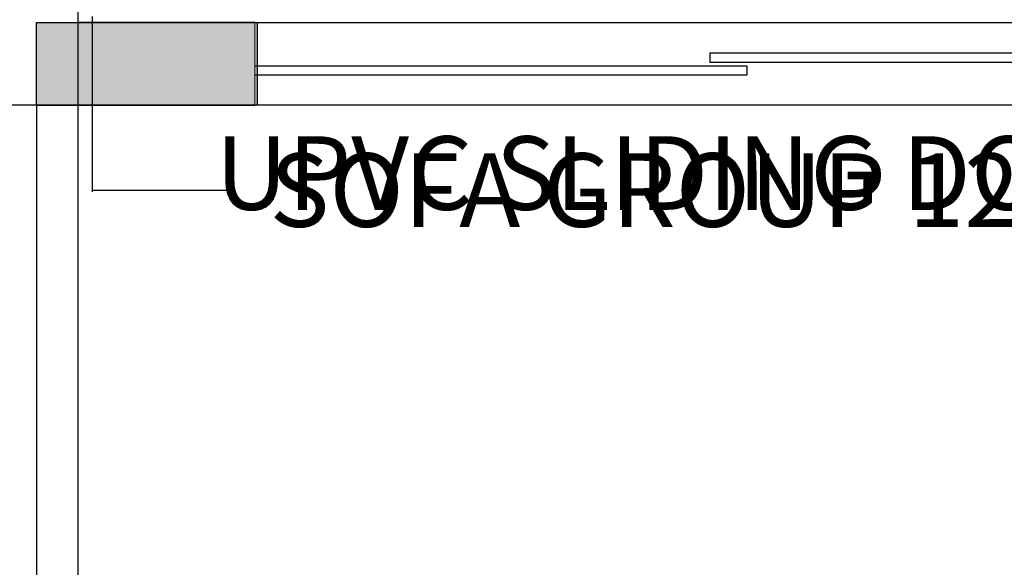
# Model space of a CAD drawing. Units: inches. Extents: x -48 to 50072, y 0 to 21068.
# Tile 47 of 75: x 16 to 123, y 628 to 687. Entities that reach past the tile are written whole.
import ezdxf

# ---------------------------------------------------------------- set-up
doc = ezdxf.new("R2010")
doc.units = ezdxf.units.IN
doc.header["$MEASUREMENT"] = 0
doc.linetypes.add('ACAD_ISO02W100', pattern=[15, 12, -3])
for name, color, linetype, lineweight in [('A-ANNO-DIMS', 2, 'Continuous', 18), ('A-ANNO-TEXT', 7, 'Continuous', 18), ('A-COLS', 1, 'Continuous', 35), ('A-DOOR', 4, 'Continuous', 18), ('A-WALL', 7, 'Continuous', 35), ('C-PROP', 7, 'Continuous', 25), ('C-PROP-REF', 32, 'ACAD_ISO02W100', 13)]:
    doc.layers.add(name, color=color, linetype=linetype, lineweight=lineweight)
doc.layers.add('Layer3', color=176, linetype='Continuous')
doc.styles.get("Standard").update_dxf_attribs({"font": 'arial.ttf'})
doc.dimstyles.get("Standard").update_dxf_attribs({"dimtxt": 8, "dimasz": 0.18, "dimexe": 0.18, "dimexo": 0.0625, "dimgap": 0.09, "dimtad": 0, "dimtih": 1, "dimtoh": 1, "dimdec": 1, "dimzin": 0, "dimdsep": 46, "dimlunit": 4, "dimtxsty": 'Standard', "dimblk": 'ARCHTICK', "dimcen": 0.09, "dimadec": 0, "dimazin": 0, "dimtfac": 1, "dimtdec": 1, "dimtofl": 0, "dimtmove": 0, "dimatfit": 3, "dimldrblk": 'ARCHTICK', "dimfxl": 1, "dimtolj": 1, "dimtzin": 0, "dimarcsym": 0})

# ---------------------------------------------------------------- blocks, each defined once
blk = doc.blocks.new('bnniku')
at = {"layer": 'Defpoints'}
h = blk.add_hatch(color=256, dxfattribs=at)
h.dxf.hatch_style = 1
h.paths.add_polyline_path([(767.55, 1114.04), (758.55, 1114.04), (758.55, 1090.04), (767.55, 1090.04)])
for p, q in [((758.55, 1114.04), (767.55, 1114.04)), ((758.55, 1090.04), (758.55, 1114.04)), ((767.55, 1114.04), (767.55, 1090.04)), ((767.55, 1090.04), (758.55, 1090.04))]:
    blk.add_line(p, q, dxfattribs=at)
blk = doc.blocks.new('fdsghhhhhhygr')
for p, q in [((41.77, 686.77), (41.77, 677.77)), ((144.77, 677.77), (144.77, 686.77))]:
    blk.add_line(p, q)
at = {"layer": 'Defpoints'}
for p, q in [((91.27, 683.47), (144.77, 683.47)), ((91.27, 683.47), (91.27, 682.47)), ((41.77, 682.07), (95.27, 682.07)), ((91.27, 682.47), (144.77, 682.47)), ((95.27, 682.07), (95.27, 681.07)), ((41.77, 681.07), (95.27, 681.07))]:
    blk.add_line(p, q, dxfattribs=at)
at = {"layer": 'Layer3'}
for p, q in [((41.77, 686.77), (144.77, 686.77)), ((144.77, 677.77), (41.77, 677.77))]:
    blk.add_line(p, q, dxfattribs=at)
blk = doc.blocks.new('_ArchTick')
at = {"color": 0, "linetype": 'ByBlock', "const_width": 0.15}
blk.add_lwpolyline([(-0.5, -0.5), (0.5, 0.5)], dxfattribs=at)
blk = doc.blocks.new('*D104')
at = {"layer": 'A-ANNO-DIMS', "color": 0, "lineweight": -2, "transparency": 16777216}
for p, q in [((51.57, 714.9), (55.29, 714.9)), ((55.11, 714.9), (55.11, 707.12)), ((55.11, 690.9), (55.11, 698.67)), ((51.57, 690.9), (55.29, 690.9))]:
    blk.add_line(p, q, dxfattribs=at)
at = {"layer": 'Defpoints', "color": 0, "transparency": 16777216}
for p in [(51.51, 714.9), (55.11, 714.9), (51.51, 690.9)]:
    blk.add_point(p, dxfattribs=at)
at = {"layer": 'A-ANNO-DIMS', "color": 0, "lineweight": -2, "transparency": 16777216, "xscale": 0.18, "yscale": 0.18, "zscale": 0.18}
for p, rotation in [((55.11, 714.9), 90), ((55.11, 690.9), 270)]:
    blk.add_blockref('_ArchTick', p, dxfattribs=dict(at, rotation=rotation))
at = {"layer": 'A-ANNO-DIMS', "color": 0, "transparency": 16777216, "insert": (55.11, 702.9), "char_height": 8, "attachment_point": 5}
blk.add_mtext('\\A1;SIDE TABLE 24', dxfattribs=at)
blk = doc.blocks.new('*D108')
at = {"layer": 'A-ANNO-DIMS', "color": 0, "lineweight": -2, "transparency": 16777216}
for p, q in [((24.1, 687.42), (24.1, 668.37)), ((150.3, 687.42), (150.3, 668.37)), ((24.1, 668.55), (39.48, 668.55)), ((150.3, 668.55), (134.91, 668.55))]:
    blk.add_line(p, q, dxfattribs=at)
at = {"layer": 'Defpoints', "color": 0, "transparency": 16777216}
for p in [(24.1, 687.48), (150.3, 687.48), (24.1, 668.55)]:
    blk.add_point(p, dxfattribs=at)
at = {"layer": 'A-ANNO-DIMS', "color": 0, "lineweight": -2, "transparency": 16777216, "xscale": 0.18, "yscale": 0.18, "zscale": 0.18, "rotation": 180}
blk.add_blockref('_ArchTick', (24.1, 668.55), dxfattribs=at)
at = {"layer": 'A-ANNO-DIMS', "color": 0, "lineweight": -2, "transparency": 16777216, "xscale": 0.18, "yscale": 0.18, "zscale": 0.18}
blk.add_blockref('_ArchTick', (150.3, 668.55), dxfattribs=at)
at = {"layer": 'A-ANNO-DIMS', "color": 0, "transparency": 16777216, "insert": (87.2, 668.55), "char_height": 8, "attachment_point": 5}
blk.add_mtext('\\A1;SOFA GROUP 126', dxfattribs=at)
blk = doc.blocks.new('*D116')
at = {"layer": 'A-ANNO-DIMS', "color": 0, "lineweight": -2, "transparency": 16777216}
for p, q in [((18.02, 677.71), (18.02, 165.94)), ((216.02, 677.71), (216.02, 165.94)), ((18.02, 166.12), (108.46, 166.12)), ((216.02, 166.12), (125.58, 166.12))]:
    blk.add_line(p, q, dxfattribs=at)
at = {"layer": 'Defpoints', "color": 0, "transparency": 16777216}
for p in [(18.02, 677.77), (216.02, 677.77), (216.02, 166.12)]:
    blk.add_point(p, dxfattribs=at)
at = {"layer": 'A-ANNO-DIMS', "color": 0, "lineweight": -2, "transparency": 16777216, "xscale": 0.18, "yscale": 0.18, "zscale": 0.18, "rotation": 180}
blk.add_blockref('_ArchTick', (18.02, 166.12), dxfattribs=at)
at = {"layer": 'A-ANNO-DIMS', "color": 0, "lineweight": -2, "transparency": 16777216, "xscale": 0.18, "yscale": 0.18, "zscale": 0.18}
blk.add_blockref('_ArchTick', (216.02, 166.12), dxfattribs=at)
at = {"layer": 'A-ANNO-DIMS', "color": 0, "transparency": 16777216, "insert": (117.02, 166.12), "char_height": 8, "attachment_point": 5}
blk.add_mtext('\\A1;198', dxfattribs=at)
blk = doc.blocks.new('*D127')
at = {"layer": 'A-ANNO-DIMS', "color": 0, "lineweight": -2, "transparency": 16777216}
for p, q in [((215.95, 677.77), (-34.61, 677.77)), ((-34.43, 677.77), (-34.43, 587.45)), ((-34.43, 488.77), (-34.43, 579.1)), ((215.95, 488.77), (-34.61, 488.77))]:
    blk.add_line(p, q, dxfattribs=at)
at = {"layer": 'Defpoints', "color": 0, "transparency": 16777216}
for p in [(-34.43, 677.77), (216.02, 677.77), (216.02, 488.77)]:
    blk.add_point(p, dxfattribs=at)
at = {"layer": 'A-ANNO-DIMS', "color": 0, "lineweight": -2, "transparency": 16777216, "xscale": 0.18, "yscale": 0.18, "zscale": 0.18}
for p, rotation in [((-34.43, 677.77), 90), ((-34.43, 488.77), 270)]:
    blk.add_blockref('_ArchTick', p, dxfattribs=dict(at, rotation=rotation))
at = {"layer": 'A-ANNO-DIMS', "color": 0, "transparency": 16777216, "insert": (-34.43, 583.27), "char_height": 8, "attachment_point": 5}
blk.add_mtext('\\A1;189', dxfattribs=at)

msp = doc.modelspace()

# ---------------------------------------------------------------- linework, layer by layer
at = {"layer": 'A-WALL'}
for p, q in [((41.766, 686.775), (22.517, 686.775)), ((41.766, 677.775), (18.017, 677.775))]:
    msp.add_line(p, q, dxfattribs=at)
at = {"layer": 'C-PROP'}
msp.add_line((22.517, 860.775), (22.517, 223.075), dxfattribs=at)
at = {"layer": 'C-PROP-REF'}
msp.add_line((18.017, 1166.275), (18.017, 214.075), dxfattribs=at)

# ---------------------------------------------------------------- block references
at = {"layer": 'A-COLS', "rotation": 90}
msp.add_blockref('bnniku', (1132.054, -80.777), dxfattribs=at)
at = {"layer": 'A-DOOR'}
msp.add_blockref('fdsghhhhhhygr', (0, 0), dxfattribs=at)

# ---------------------------------------------------------------- texts
at = {"layer": 'A-ANNO-TEXT', "insert": (37.479, 674.399), "char_height": 8, "attachment_point": 1}
msp.add_mtext_dynamic_manual_height_columns('UPVC SLIDING DOOR ', width=126.59735, gutter_width=40, heights=[0], dxfattribs=at)

# ---------------------------------------------------------------- dimensions: what is measured, and where the dimension line sits
at = {"layer": 'A-ANNO-DIMS'}
for base, p1, p2, angle, text, picture, middle in [((55.11, 714.897), (51.51, 690.897), (51.51, 714.897), 90, 'SIDE TABLE <>', '*D104', (55.11, 702.897)), ((24.097, 668.554), (150.298, 687.484), (24.097, 687.484), 180, 'SOFA GROUP <>', '*D108', (87.197, 668.554))]:
    dim = msp.add_linear_dim(base=base, p1=p1, p2=p2, angle=angle, text=text, dimstyle='Standard', override={"dimdec": 0, "dimlfac": 1, "dimrnd": 0, "dimzin": 0, "dimdsep": 46, "dimlunit": 2}, dxfattribs=at)
    dim.commit()
    dim.dimension.update_dxf_attribs({"geometry": picture, "text_midpoint": middle})
dim = msp.add_linear_dim(base=(-34.433, 677.775), p1=(216.017, 488.775), p2=(216.017, 677.775), angle=90, dimstyle='Standard', override={"dimdec": 0, "dimlfac": 1, "dimrnd": 0, "dimzin": 0, "dimdsep": 46, "dimlunit": 2}, dxfattribs=at)
dim.commit()
dim.dimension.update_dxf_attribs({"geometry": '*D127', "text_midpoint": (-34.433, 583.275)})
dim = msp.add_linear_dim(base=(216.017, 166.125), p1=(18.017, 677.775), p2=(216.017, 677.775), dimstyle='Standard', override={"dimdec": 0, "dimlfac": 1, "dimrnd": 0, "dimzin": 0, "dimdsep": 46, "dimlunit": 2}, dxfattribs=at)
dim.commit()
dim.dimension.update_dxf_attribs({"geometry": '*D116', "text_midpoint": (117.017, 166.125)})

doc.saveas('drawing.dxf')
